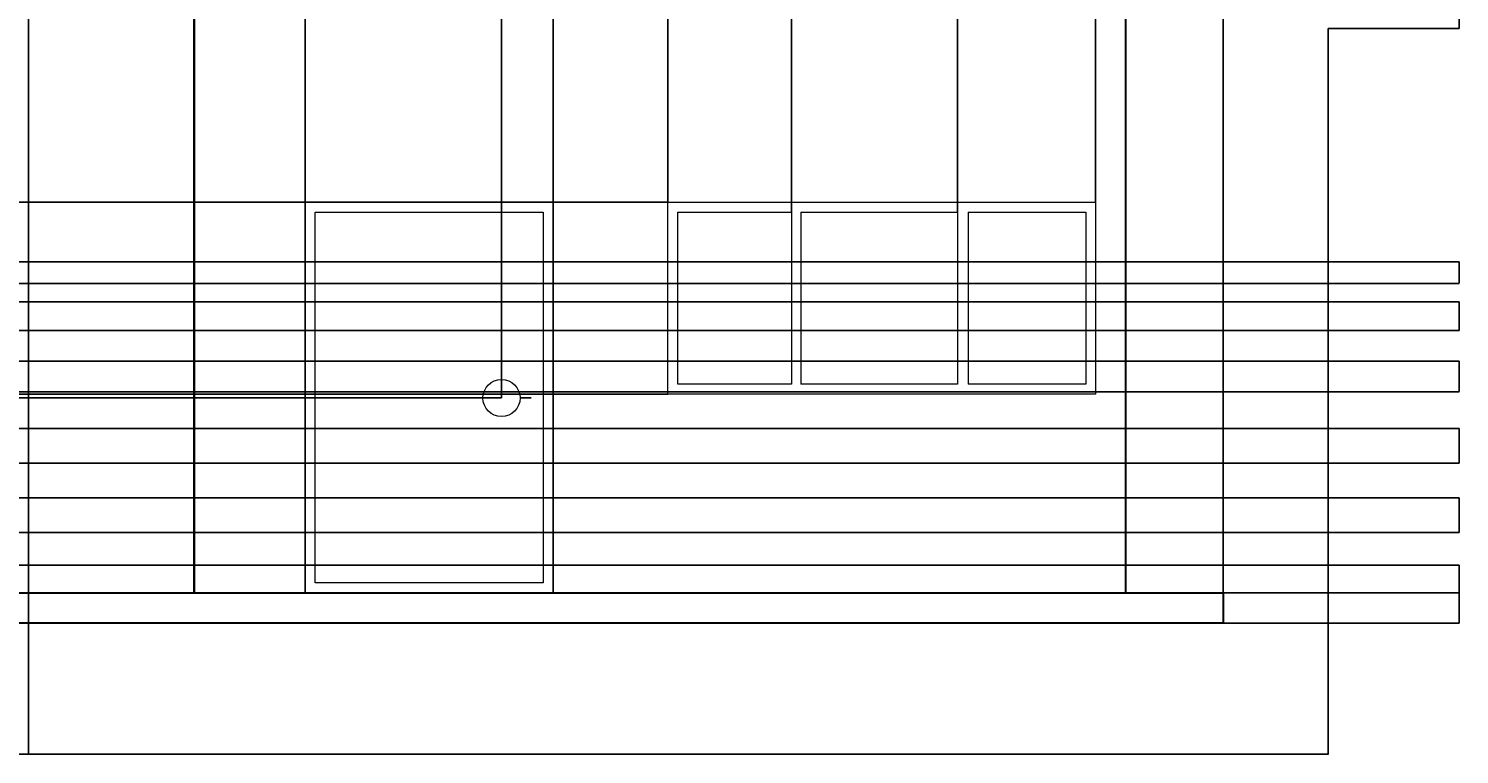
# Model space of a CAD drawing. Units: millimetres. Extents: x 1225 to 9865, y 11 to 4912.
# Tile 3 of 4: x 5562 to 9865, y 11 to 2192. Entities that reach past the tile are written whole.
import ezdxf

# ---------------------------------------------------------------- set-up
doc = ezdxf.new("R2010")
doc.units = ezdxf.units.MM
for name, color, linetype, lineweight in [('A-ANNO-DIMS', 2, 'Continuous', 18), ('A-COLS', 7, 'Continuous', 35), ('A-DOOR', 3, 'Continuous', 20), ('A-GLAZ', 4, 'Continuous', 18), ('A-WALL', 7, 'Continuous', 30), ('S-FNDN', 7, 'Continuous', 30)]:
    doc.layers.add(name, color=color, linetype=linetype, lineweight=lineweight)
doc.styles.get("Standard").update_dxf_attribs({"font": 'arial.ttf'})
doc.dimstyles.get("Standard").update_dxf_attribs({"dimtxt": 0.18, "dimasz": 0.18, "dimexe": 0.18, "dimexo": 0.0625, "dimgap": 0.09, "dimtad": 0, "dimtih": 1, "dimtoh": 1, "dimdec": 4, "dimzin": 0, "dimdsep": 46, "dimtxsty": 'Standard', "dimcen": 0.09, "dimadec": 0, "dimazin": 0, "dimtfac": 1, "dimtdec": 4, "dimtofl": 0, "dimtmove": 0, "dimatfit": 3, "dimfxl": 1, "dimtolj": 1, "dimtzin": 0, "dimarcsym": 0})

# ---------------------------------------------------------------- blocks, each defined once
blk = doc.blocks.new('*D1')
at = {"layer": 'A-ANNO-DIMS', "color": 0, "lineweight": -2, "transparency": 16777216}
for p, q in [((9470.3, 2192.1), (9470.3, 10.6)), ((1619.2, 404.7), (1619.2, 10.6)), ((1619.3, 10.8), (5544.4, 10.8)), ((9470.1, 10.8), (5545.1, 10.8))]:
    blk.add_line(p, q, dxfattribs=at)
at = {"layer": 'A-ANNO-DIMS', "color": 0, "transparency": 16777216}
for points in [[(1619.3, 10.8), (1619.3, 10.7), (1619.2, 10.8)], [(9470.1, 10.8), (9470.1, 10.7), (9470.3, 10.8)]]:
    blk.add_solid(points, dxfattribs=at)
at = {"layer": 'Defpoints', "color": 0, "transparency": 16777216}
for p in [(9470.3, 2192.2), (1619.2, 404.8), (9470.3, 10.8)]:
    blk.add_point(p, dxfattribs=at)
at = {"layer": 'A-ANNO-DIMS', "color": 0, "transparency": 16777216, "insert": (5544.7, 10.8), "char_height": 0.18, "attachment_point": 5}
blk.add_mtext('\\A1;7851', dxfattribs=at)
blk = doc.blocks.new('*D9')
at = {"layer": 'A-ANNO-DIMS', "color": 0, "lineweight": -2, "transparency": 16777216}
for p, q in [((5415.4, 4322.4), (5415.4, 10.6)), ((5561.8, 4322.4), (5561.8, 10.6)), ((5415.6, 10.8), (5488.1, 10.8)), ((5561.6, 10.8), (5489, 10.8))]:
    blk.add_line(p, q, dxfattribs=at)
at = {"layer": 'A-ANNO-DIMS', "color": 0, "transparency": 16777216}
for points in [[(5415.6, 10.8), (5415.6, 10.7), (5415.4, 10.8)], [(5561.6, 10.8), (5561.6, 10.7), (5561.8, 10.8)]]:
    blk.add_solid(points, dxfattribs=at)
at = {"layer": 'Defpoints', "color": 0, "transparency": 16777216}
for p in [(5415.4, 4322.4), (5561.8, 4322.4), (5561.8, 10.8)]:
    blk.add_point(p, dxfattribs=at)
at = {"layer": 'A-ANNO-DIMS', "color": 0, "transparency": 16777216, "insert": (5488.6, 10.8), "char_height": 0.18, "attachment_point": 5}
blk.add_mtext('\\A1;146.38', dxfattribs=at)
blk = doc.blocks.new('*D12')
at = {"layer": 'A-ANNO-DIMS', "color": 0, "lineweight": -2, "transparency": 16777216}
for p, q in [((6059.9, 496.3), (6059.9, 4911.8)), ((6060.1, 4911.6), (6226, 4911.6)), ((6392.9, 4911.6), (6226.9, 4911.6)), ((6393.1, 496.3), (6393.1, 4911.8))]:
    blk.add_line(p, q, dxfattribs=at)
at = {"layer": 'A-ANNO-DIMS', "color": 0, "transparency": 16777216}
for points in [[(6060.1, 4911.6), (6060.1, 4911.6), (6059.9, 4911.6)], [(6392.9, 4911.6), (6392.9, 4911.6), (6393.1, 4911.6)]]:
    blk.add_solid(points, dxfattribs=at)
at = {"layer": 'Defpoints', "color": 0, "transparency": 16777216}
for p in [(6393.1, 4911.6), (6059.9, 496.3), (6393.1, 496.3)]:
    blk.add_point(p, dxfattribs=at)
at = {"layer": 'A-ANNO-DIMS', "color": 0, "transparency": 16777216, "insert": (6226.5, 4911.6), "char_height": 0.18, "attachment_point": 5}
blk.add_mtext('\\A1;333.14', dxfattribs=at)
blk = doc.blocks.new('*D13')
at = {"layer": 'A-ANNO-DIMS', "color": 0, "lineweight": -2, "transparency": 16777216}
for p, q in [((6393.1, 1670.9), (6393.1, 4911.8)), ((6393.2, 4911.6), (6765.6, 4911.6)), ((7138.7, 4911.6), (6766.3, 4911.6)), ((7138.8, 1670.9), (7138.8, 4911.8))]:
    blk.add_line(p, q, dxfattribs=at)
at = {"layer": 'A-ANNO-DIMS', "color": 0, "transparency": 16777216}
for points in [[(6393.2, 4911.6), (6393.2, 4911.6), (6393.1, 4911.6)], [(7138.7, 4911.6), (7138.7, 4911.6), (7138.8, 4911.6)]]:
    blk.add_solid(points, dxfattribs=at)
at = {"layer": 'Defpoints', "color": 0, "transparency": 16777216}
for p in [(7138.8, 4911.6), (6393.1, 1670.8), (7138.8, 1670.8)]:
    blk.add_point(p, dxfattribs=at)
at = {"layer": 'A-ANNO-DIMS', "color": 0, "transparency": 16777216, "insert": (6765.9, 4911.6), "char_height": 0.18, "attachment_point": 5}
blk.add_mtext('\\A1;745.8', dxfattribs=at)
blk = doc.blocks.new('*D14')
at = {"layer": 'A-ANNO-DIMS', "color": 0, "lineweight": -2, "transparency": 16777216}
for p, q in [((6983.8, 1082), (6983.8, 4911.8)), ((6984, 4911.6), (7061.1, 4911.6)), ((7138.7, 4911.6), (7061.6, 4911.6)), ((7138.8, 496.3), (7138.8, 4911.8))]:
    blk.add_line(p, q, dxfattribs=at)
at = {"layer": 'A-ANNO-DIMS', "color": 0, "transparency": 16777216}
for points in [[(6984, 4911.6), (6984, 4911.6), (6983.8, 4911.6)], [(7138.7, 4911.6), (7138.7, 4911.6), (7138.8, 4911.6)]]:
    blk.add_solid(points, dxfattribs=at)
at = {"layer": 'Defpoints', "color": 0, "transparency": 16777216}
for p in [(7138.8, 4911.6), (6983.8, 1081.9), (7138.8, 496.3)]:
    blk.add_point(p, dxfattribs=at)
at = {"layer": 'A-ANNO-DIMS', "color": 0, "transparency": 16777216, "insert": (7061.3, 4911.6), "char_height": 0.18, "attachment_point": 5}
blk.add_mtext('\\A1;155', dxfattribs=at)
blk = doc.blocks.new('*D15')
at = {"layer": 'A-ANNO-DIMS', "color": 0, "lineweight": -2, "transparency": 16777216}
for p, q in [((7138.8, 1670.9), (7138.8, 4911.8)), ((7139, 4911.6), (7311.1, 4911.6)), ((7484.1, 4911.6), (7311.9, 4911.6)), ((7484.2, 1670.9), (7484.2, 4911.8))]:
    blk.add_line(p, q, dxfattribs=at)
at = {"layer": 'A-ANNO-DIMS', "color": 0, "transparency": 16777216}
for points in [[(7139, 4911.6), (7139, 4911.6), (7138.8, 4911.6)], [(7484.1, 4911.6), (7484.1, 4911.6), (7484.2, 4911.6)]]:
    blk.add_solid(points, dxfattribs=at)
at = {"layer": 'Defpoints', "color": 0, "transparency": 16777216}
for p in [(7484.2, 4911.6), (7138.8, 1670.8), (7484.2, 1670.8)]:
    blk.add_point(p, dxfattribs=at)
at = {"layer": 'A-ANNO-DIMS', "color": 0, "transparency": 16777216, "insert": (7311.5, 4911.6), "char_height": 0.18, "attachment_point": 5}
blk.add_mtext('\\A1;345.4', dxfattribs=at)
blk = doc.blocks.new('*D16')
at = {"layer": 'A-ANNO-DIMS', "color": 0, "lineweight": -2, "transparency": 16777216}
for p, q in [((8861.3, 496.3), (8861.3, 4911.8)), ((8861.4, 4911.6), (9007.3, 4911.6)), ((9153.9, 4911.6), (9008.1, 4911.6)), ((9154.1, 496.3), (9154.1, 4911.8))]:
    blk.add_line(p, q, dxfattribs=at)
at = {"layer": 'A-ANNO-DIMS', "color": 0, "transparency": 16777216}
for points in [[(8861.4, 4911.6), (8861.4, 4911.6), (8861.3, 4911.6)], [(9153.9, 4911.6), (9153.9, 4911.6), (9154.1, 4911.6)]]:
    blk.add_solid(points, dxfattribs=at)
at = {"layer": 'Defpoints', "color": 0, "transparency": 16777216}
for p in [(9154.1, 4911.6), (8861.3, 496.3), (9154.1, 496.3)]:
    blk.add_point(p, dxfattribs=at)
at = {"layer": 'A-ANNO-DIMS', "color": 0, "transparency": 16777216, "insert": (9007.7, 4911.6), "char_height": 0.18, "attachment_point": 5}
blk.add_mtext('\\A1;292.8', dxfattribs=at)
blk = doc.blocks.new('*D26')
at = {"layer": 'A-ANNO-DIMS', "color": 0, "lineweight": -2, "transparency": 16777216}
for p, q in [((9154.1, 496.3), (9864.4, 496.3)), ((9864.3, 496.1), (9864.3, 450.7)), ((9864.3, 404.9), (9864.3, 450.3)), ((9154.1, 404.8), (9864.4, 404.8))]:
    blk.add_line(p, q, dxfattribs=at)
at = {"layer": 'A-ANNO-DIMS', "color": 0, "transparency": 16777216}
for points in [[(9864.2, 496.1), (9864.3, 496.1), (9864.3, 496.3)], [(9864.2, 404.9), (9864.3, 404.9), (9864.3, 404.8)]]:
    blk.add_solid(points, dxfattribs=at)
at = {"layer": 'Defpoints', "color": 0, "transparency": 16777216}
for p in [(9154.1, 496.3), (9864.3, 496.3), (9154.1, 404.8)]:
    blk.add_point(p, dxfattribs=at)
at = {"layer": 'A-ANNO-DIMS', "color": 0, "transparency": 16777216, "insert": (9864.3, 450.5), "char_height": 0.18, "attachment_point": 5}
blk.add_mtext('\\A1;91.51', dxfattribs=at)
blk = doc.blocks.new('*D30')
at = {"layer": 'A-ANNO-DIMS', "color": 0, "lineweight": -2, "transparency": 16777216}
for p, q in [((9470.3, 2343), (9864.4, 2343)), ((9864.3, 2342.8), (9864.3, 2267.8)), ((9864.3, 2192.3), (9864.3, 2267.4)), ((9470.3, 2192.2), (9864.4, 2192.2))]:
    blk.add_line(p, q, dxfattribs=at)
at = {"layer": 'A-ANNO-DIMS', "color": 0, "transparency": 16777216}
for points in [[(9864.2, 2342.8), (9864.3, 2342.8), (9864.3, 2343)], [(9864.2, 2192.3), (9864.3, 2192.3), (9864.3, 2192.2)]]:
    blk.add_solid(points, dxfattribs=at)
at = {"layer": 'Defpoints', "color": 0, "transparency": 16777216}
for p in [(9470.3, 2343), (9864.3, 2343), (9470.3, 2192.2)]:
    blk.add_point(p, dxfattribs=at)
at = {"layer": 'A-ANNO-DIMS', "color": 0, "transparency": 16777216, "insert": (9864.3, 2267.6), "char_height": 0.18, "attachment_point": 5}
blk.add_mtext('\\A1;150.8', dxfattribs=at)
blk = doc.blocks.new('*D38')
at = {"layer": 'A-ANNO-DIMS', "color": 0, "lineweight": -2, "transparency": 16777216}
for p, q in [((6393, 1670.8), (1225, 1670.8)), ((1225.2, 1670.7), (1225.2, 1083.7)), ((1225.2, 496.4), (1225.2, 1083.4)), ((6393, 496.3), (1225, 496.3))]:
    blk.add_line(p, q, dxfattribs=at)
at = {"layer": 'A-ANNO-DIMS', "color": 0, "transparency": 16777216}
for points in [[(1225.1, 1670.7), (1225.2, 1670.7), (1225.2, 1670.8)], [(1225.1, 496.4), (1225.2, 496.4), (1225.2, 496.3)]]:
    blk.add_solid(points, dxfattribs=at)
at = {"layer": 'Defpoints', "color": 0, "transparency": 16777216}
for p in [(1225.2, 1670.8), (6393.1, 1670.8), (6393.1, 496.3)]:
    blk.add_point(p, dxfattribs=at)
at = {"layer": 'A-ANNO-DIMS', "color": 0, "transparency": 16777216, "insert": (1225.2, 1083.6), "char_height": 0.18, "attachment_point": 5}
blk.add_mtext('\\A1;1174.6', dxfattribs=at)
blk = doc.blocks.new('*D39')
at = {"layer": 'A-ANNO-DIMS', "color": 0, "lineweight": -2, "transparency": 16777216}
for p, q in [((7484.2, 1670.8), (1225, 1670.8)), ((1225.2, 1670.7), (1225.2, 1382.4)), ((1225.2, 1093.8), (1225.2, 1382.1)), ((7484.2, 1093.7), (1225, 1093.7))]:
    blk.add_line(p, q, dxfattribs=at)
at = {"layer": 'A-ANNO-DIMS', "color": 0, "transparency": 16777216}
for points in [[(1225.1, 1670.7), (1225.2, 1670.7), (1225.2, 1670.8)], [(1225.1, 1093.8), (1225.2, 1093.8), (1225.2, 1093.7)]]:
    blk.add_solid(points, dxfattribs=at)
at = {"layer": 'Defpoints', "color": 0, "transparency": 16777216}
for p in [(1225.2, 1670.8), (7484.2, 1670.8), (7484.2, 1093.7)]:
    blk.add_point(p, dxfattribs=at)
at = {"layer": 'A-ANNO-DIMS', "color": 0, "transparency": 16777216, "insert": (1225.2, 1382.3), "char_height": 0.18, "attachment_point": 5}
blk.add_mtext('\\A1;577.2', dxfattribs=at)
blk = doc.blocks.new('*D44')
at = {"layer": 'A-ANNO-DIMS', "color": 0, "lineweight": -2, "transparency": 16777216}
for p, q in [((6983.8, 1081.9), (1225, 1081.9)), ((1225.2, 1081.8), (1225.2, 789.3)), ((1225.2, 496.4), (1225.2, 788.9)), ((7138.8, 496.3), (1225, 496.3))]:
    blk.add_line(p, q, dxfattribs=at)
at = {"layer": 'A-ANNO-DIMS', "color": 0, "transparency": 16777216}
for points in [[(1225.1, 1081.8), (1225.2, 1081.8), (1225.2, 1081.9)], [(1225.1, 496.4), (1225.2, 496.4), (1225.2, 496.3)]]:
    blk.add_solid(points, dxfattribs=at)
at = {"layer": 'Defpoints', "color": 0, "transparency": 16777216}
for p in [(6983.8, 1081.9), (1225.2, 496.3), (7138.8, 496.3)]:
    blk.add_point(p, dxfattribs=at)
at = {"layer": 'A-ANNO-DIMS', "color": 0, "transparency": 16777216, "insert": (1225.2, 789.1), "char_height": 0.18, "attachment_point": 5}
blk.add_mtext('\\A1;585.7', dxfattribs=at)
blk = doc.blocks.new('*D52')
at = {"layer": 'A-ANNO-DIMS', "color": 0, "lineweight": -2, "transparency": 16777216}
for p, q in [((7484.2, 1670.9), (7484.2, 4911.8)), ((7484.4, 4911.6), (7670, 4911.6)), ((7856.1, 4911.6), (7670.5, 4911.6)), ((7856.2, 1640.9), (7856.2, 4911.8))]:
    blk.add_line(p, q, dxfattribs=at)
at = {"layer": 'A-ANNO-DIMS', "color": 0, "transparency": 16777216}
for points in [[(7484.4, 4911.6), (7484.4, 4911.6), (7484.2, 4911.6)], [(7856.1, 4911.6), (7856.1, 4911.6), (7856.2, 4911.6)]]:
    blk.add_solid(points, dxfattribs=at)
at = {"layer": 'Defpoints', "color": 0, "transparency": 16777216}
for p in [(7856.2, 4911.6), (7484.2, 1670.8), (7856.2, 1640.8)]:
    blk.add_point(p, dxfattribs=at)
at = {"layer": 'A-ANNO-DIMS', "color": 0, "transparency": 16777216, "insert": (7670.2, 4911.6), "char_height": 0.18, "attachment_point": 5}
blk.add_mtext('\\A1;372', dxfattribs=at)
blk = doc.blocks.new('*D53')
at = {"layer": 'A-ANNO-DIMS', "color": 0, "lineweight": -2, "transparency": 16777216}
for p, q in [((7856.2, 1640.9), (7856.2, 4911.8)), ((7856.4, 4911.6), (8105.4, 4911.6)), ((8355.2, 4911.6), (8106.2, 4911.6)), ((8355.4, 1640.9), (8355.4, 4911.8))]:
    blk.add_line(p, q, dxfattribs=at)
at = {"layer": 'A-ANNO-DIMS', "color": 0, "transparency": 16777216}
for points in [[(7856.4, 4911.6), (7856.4, 4911.6), (7856.2, 4911.6)], [(8355.2, 4911.6), (8355.2, 4911.6), (8355.4, 4911.6)]]:
    blk.add_solid(points, dxfattribs=at)
at = {"layer": 'Defpoints', "color": 0, "transparency": 16777216}
for p in [(8355.4, 4911.6), (7856.2, 1640.8), (8355.4, 1640.8)]:
    blk.add_point(p, dxfattribs=at)
at = {"layer": 'A-ANNO-DIMS', "color": 0, "transparency": 16777216, "insert": (8105.8, 4911.6), "char_height": 0.18, "attachment_point": 5}
blk.add_mtext('\\A1;499.1', dxfattribs=at)
blk = doc.blocks.new('*D54')
at = {"layer": 'A-ANNO-DIMS', "color": 0, "lineweight": -2, "transparency": 16777216}
for p, q in [((8355.4, 1640.9), (8355.4, 4911.8)), ((8355.5, 4911.6), (8562.6, 4911.6)), ((8770.5, 4911.6), (8563.5, 4911.6)), ((8770.7, 1670.9), (8770.7, 4911.8))]:
    blk.add_line(p, q, dxfattribs=at)
at = {"layer": 'A-ANNO-DIMS', "color": 0, "transparency": 16777216}
for points in [[(8355.5, 4911.6), (8355.5, 4911.6), (8355.4, 4911.6)], [(8770.5, 4911.6), (8770.5, 4911.6), (8770.7, 4911.6)]]:
    blk.add_solid(points, dxfattribs=at)
at = {"layer": 'Defpoints', "color": 0, "transparency": 16777216}
for p in [(8770.7, 4911.6), (8355.4, 1640.8), (8770.7, 1670.8)]:
    blk.add_point(p, dxfattribs=at)
at = {"layer": 'A-ANNO-DIMS', "color": 0, "transparency": 16777216, "insert": (8563, 4911.6), "char_height": 0.18, "attachment_point": 5}
blk.add_mtext('\\A1;415.36', dxfattribs=at)
blk = doc.blocks.new('*D67')
at = {"layer": 'A-ANNO-DIMS', "color": 0, "lineweight": -2, "transparency": 16777216}
for p, q in [((4013.7, 579.2), (9864.4, 579.2)), ((9864.3, 579), (9864.3, 537.9)), ((9864.3, 496.4), (9864.3, 537.6)), ((4013.7, 496.3), (9864.4, 496.3))]:
    blk.add_line(p, q, dxfattribs=at)
at = {"layer": 'A-ANNO-DIMS', "color": 0, "transparency": 16777216}
for points in [[(9864.2, 579), (9864.3, 579), (9864.3, 579.2)], [(9864.2, 496.4), (9864.3, 496.4), (9864.3, 496.3)]]:
    blk.add_solid(points, dxfattribs=at)
at = {"layer": 'Defpoints', "color": 0, "transparency": 16777216}
for p in [(4013.6, 579.2), (9864.3, 579.2), (4013.6, 496.3)]:
    blk.add_point(p, dxfattribs=at)
at = {"layer": 'A-ANNO-DIMS', "color": 0, "transparency": 16777216, "insert": (9864.3, 537.7), "char_height": 0.18, "attachment_point": 5}
blk.add_mtext('\\A1;82.96', dxfattribs=at)
blk = doc.blocks.new('*D68')
at = {"layer": 'A-ANNO-DIMS', "color": 0, "lineweight": -2, "transparency": 16777216}
for p, q in [((4013.7, 781.7), (9864.4, 781.7)), ((9864.3, 781.5), (9864.3, 729.7)), ((9864.3, 677.6), (9864.3, 729.4)), ((4013.7, 677.4), (9864.4, 677.4))]:
    blk.add_line(p, q, dxfattribs=at)
at = {"layer": 'A-ANNO-DIMS', "color": 0, "transparency": 16777216}
for points in [[(9864.2, 781.5), (9864.3, 781.5), (9864.3, 781.7)], [(9864.2, 677.6), (9864.3, 677.6), (9864.3, 677.4)]]:
    blk.add_solid(points, dxfattribs=at)
at = {"layer": 'Defpoints', "color": 0, "transparency": 16777216}
for p in [(4013.6, 781.7), (9864.3, 781.7), (4013.6, 677.4)]:
    blk.add_point(p, dxfattribs=at)
at = {"layer": 'A-ANNO-DIMS', "color": 0, "transparency": 16777216, "insert": (9864.3, 729.5), "char_height": 0.18, "attachment_point": 5}
blk.add_mtext('\\A1;104.3', dxfattribs=at)
blk = doc.blocks.new('*D69')
at = {"layer": 'A-ANNO-DIMS', "color": 0, "lineweight": -2, "transparency": 16777216}
for p, q in [((4013.7, 990.3), (9864.4, 990.3)), ((9864.3, 990.1), (9864.3, 938.3)), ((9864.3, 886.2), (9864.3, 938)), ((4013.7, 886), (9864.4, 886))]:
    blk.add_line(p, q, dxfattribs=at)
at = {"layer": 'A-ANNO-DIMS', "color": 0, "transparency": 16777216}
for points in [[(9864.2, 990.1), (9864.3, 990.1), (9864.3, 990.3)], [(9864.2, 886.2), (9864.3, 886.2), (9864.3, 886)]]:
    blk.add_solid(points, dxfattribs=at)
at = {"layer": 'Defpoints', "color": 0, "transparency": 16777216}
for p in [(4013.6, 990.3), (9864.3, 990.3), (4013.6, 886)]:
    blk.add_point(p, dxfattribs=at)
at = {"layer": 'A-ANNO-DIMS', "color": 0, "transparency": 16777216, "insert": (9864.3, 938.2), "char_height": 0.18, "attachment_point": 5}
blk.add_mtext('\\A1;104.3', dxfattribs=at)
blk = doc.blocks.new('*D70')
at = {"layer": 'A-ANNO-DIMS', "color": 0, "lineweight": -2, "transparency": 16777216}
for p, q in [((4013.7, 1192.8), (9864.4, 1192.8)), ((9864.3, 1192.6), (9864.3, 1147)), ((9864.3, 1100.9), (9864.3, 1146.6)), ((4013.7, 1100.8), (9864.4, 1100.8))]:
    blk.add_line(p, q, dxfattribs=at)
at = {"layer": 'A-ANNO-DIMS', "color": 0, "transparency": 16777216}
for points in [[(9864.2, 1192.6), (9864.3, 1192.6), (9864.3, 1192.8)], [(9864.2, 1100.9), (9864.3, 1100.9), (9864.3, 1100.8)]]:
    blk.add_solid(points, dxfattribs=at)
at = {"layer": 'Defpoints', "color": 0, "transparency": 16777216}
for p in [(4013.6, 1192.8), (9864.3, 1192.8), (4013.6, 1100.8)]:
    blk.add_point(p, dxfattribs=at)
at = {"layer": 'A-ANNO-DIMS', "color": 0, "transparency": 16777216, "insert": (9864.3, 1146.8), "char_height": 0.18, "attachment_point": 5}
blk.add_mtext('\\A1;92.04', dxfattribs=at)
blk = doc.blocks.new('*D71')
at = {"layer": 'A-ANNO-DIMS', "color": 0, "lineweight": -2, "transparency": 16777216}
for p, q in [((4013.7, 1370.7), (9864.4, 1370.7)), ((9864.3, 1370.6), (9864.3, 1328)), ((9864.3, 1285), (9864.3, 1327.6)), ((4013.7, 1284.8), (9864.4, 1284.8))]:
    blk.add_line(p, q, dxfattribs=at)
at = {"layer": 'A-ANNO-DIMS', "color": 0, "transparency": 16777216}
for points in [[(9864.2, 1370.6), (9864.3, 1370.6), (9864.3, 1370.7)], [(9864.2, 1285), (9864.3, 1285), (9864.3, 1284.8)]]:
    blk.add_solid(points, dxfattribs=at)
at = {"layer": 'Defpoints', "color": 0, "transparency": 16777216}
for p in [(4013.6, 1370.7), (9864.3, 1370.7), (4013.6, 1284.8)]:
    blk.add_point(p, dxfattribs=at)
at = {"layer": 'A-ANNO-DIMS', "color": 0, "transparency": 16777216, "insert": (9864.3, 1327.8), "char_height": 0.18, "attachment_point": 5}
blk.add_mtext('\\A1;85.9', dxfattribs=at)
blk = doc.blocks.new('*D72')
at = {"layer": 'A-ANNO-DIMS', "color": 0, "lineweight": -2, "transparency": 16777216}
for p, q in [((4013.7, 1491.5), (9864.4, 1491.5)), ((9864.3, 1491.4), (9864.3, 1459.1)), ((4013.7, 1426.4), (9864.4, 1426.4)), ((9864.3, 1426.6), (9864.3, 1458.8))]:
    blk.add_line(p, q, dxfattribs=at)
at = {"layer": 'A-ANNO-DIMS', "color": 0, "transparency": 16777216}
for points in [[(9864.2, 1491.4), (9864.3, 1491.4), (9864.3, 1491.5)], [(9864.2, 1426.6), (9864.3, 1426.6), (9864.3, 1426.4)]]:
    blk.add_solid(points, dxfattribs=at)
at = {"layer": 'Defpoints', "color": 0, "transparency": 16777216}
for p in [(4013.6, 1491.5), (9864.3, 1491.5), (4013.6, 1426.4)]:
    blk.add_point(p, dxfattribs=at)
at = {"layer": 'A-ANNO-DIMS', "color": 0, "transparency": 16777216, "insert": (9864.3, 1459), "char_height": 0.18, "attachment_point": 5}
blk.add_mtext('\\A1;65.16', dxfattribs=at)
blk = doc.blocks.new('*D73')
at = {"layer": 'A-ANNO-DIMS', "color": 0, "lineweight": -2, "transparency": 16777216}
for p, q in [((6983.8, 1081.9), (6983.8, 1082)), ((6983.8, 1081.9), (6983.9, 1081.9)), ((7073.2, 1081.9), (7039.9, 1081.9))]:
    blk.add_line(p, q, dxfattribs=at)
at = {"layer": 'A-ANNO-DIMS', "color": 0, "transparency": 16777216}
blk.add_solid([(7039.9, 1082), (7039.9, 1081.9), (7039.7, 1081.9)], dxfattribs=at)
at = {"layer": 'Defpoints', "color": 0, "transparency": 16777216}
for p in [(6928, 1081.9), (7039.7, 1081.9)]:
    blk.add_point(p, dxfattribs=at)
at = {"layer": 'A-ANNO-DIMS', "color": 0, "transparency": 16777216, "insert": (7073.8, 1081.9), "char_height": 0.18, "attachment_point": 5}
blk.add_mtext('\\A1;∅111.74', dxfattribs=at)

msp = doc.modelspace()

# ---------------------------------------------------------------- linework, layer by layer
at = {"layer": 'A-COLS'}
msp.add_line((6059.917, 4517.596), (6059.917, 496.264), dxfattribs=at)
at = {"layer": 'A-DOOR'}
for points in [[(6393.055, 1670.836), (7138.844, 1670.836), (7138.844, 496.264), (6393.055, 496.264)], [(6423.055, 1640.836), (7108.844, 1640.836), (7108.844, 526.264), (6423.055, 526.264)]]:
    msp.add_lwpolyline(points, close=True, dxfattribs=at)
msp.add_circle((6983.847, 1081.944), 55.87, dxfattribs=at)
at = {"layer": 'A-GLAZ'}
for p, q in [((7856.234, 1640.836), (7856.234, 1123.666)), ((7884.302, 1640.836), (7884.302, 1123.666)), ((8355.362, 1640.836), (8355.362, 1123.666)), ((8387.1, 1640.836), (8387.1, 1123.666))]:
    msp.add_line(p, q, dxfattribs=at)
msp.add_lwpolyline([(7484.241, 1670.836), (8770.718, 1670.836), (8770.718, 1093.666), (7484.241, 1093.666)], close=True, dxfattribs=at)
for points in [[(7856.234, 1123.666), (7514.241, 1123.666), (7514.241, 1640.836), (7856.234, 1640.836)], [(7884.302, 1640.836), (8355.362, 1640.836)], [(8387.1, 1640.836), (8740.718, 1640.836), (8740.718, 1123.666), (8387.1, 1123.666)], [(8355.362, 1123.666), (7884.302, 1123.666)]]:
    msp.add_lwpolyline(points, dxfattribs=at)
at = {"layer": 'A-WALL'}
for p, q in [((8861.261, 496.264), (8861.261, 3844.439)), ((6059.917, 496.264), (8861.261, 496.264))]:
    msp.add_line(p, q, dxfattribs=at)
at = {"layer": 'S-FNDN'}
for p, q in [((1619.167, 496.264), (6462.269, 496.264)), ((6462.269, 496.264), (9154.083, 496.264)), ((9154.083, 496.264), (9154.083, 404.75)), ((6462.269, 404.75), (1619.167, 404.75)), ((9154.083, 404.75), (6462.269, 404.75))]:
    msp.add_line(p, q, dxfattribs=at)

# ---------------------------------------------------------------- dimensions: what is measured, and where the dimension line sits
at = {"layer": 'A-ANNO-DIMS'}
for base, p1, p2, override, picture, middle in [((6393.055, 4911.596), (6059.917, 496.264), (6393.055, 496.264), {"dimdec": 2, "dimlfac": 1, "dimrnd": 0, "dimzin": 0, "dimdsep": 46, "dimlunit": 2}, '*D12', (6226.486, 4911.596)), ((7138.844, 4911.596), (6393.055, 1670.836), (7138.844, 1670.836), {"dimdec": 1, "dimlfac": 1, "dimrnd": 0, "dimzin": 0, "dimdsep": 46, "dimlunit": 2}, '*D13', (6765.95, 4911.596)), ((7138.844, 4911.596), (6983.847, 1081.944), (7138.844, 496.264), {"dimdec": 0, "dimlfac": 1, "dimrnd": 0, "dimzin": 0, "dimdsep": 46, "dimlunit": 2}, '*D14', (7061.346, 4911.596)), ((7484.241, 4911.596), (7138.844, 1670.836), (7484.241, 1670.836), {"dimdec": 1, "dimlfac": 1, "dimrnd": 0, "dimzin": 0, "dimdsep": 46, "dimlunit": 2}, '*D15', (7311.543, 4911.596)), ((7856.234, 4911.596), (7484.241, 1670.836), (7856.234, 1640.836), {"dimdec": 0, "dimlfac": 1, "dimrnd": 0, "dimzin": 0, "dimdsep": 46, "dimlunit": 2}, '*D52', (7670.238, 4911.596)), ((8355.362, 4911.596), (7856.234, 1640.836), (8355.362, 1640.836), {"dimdec": 1, "dimlfac": 1, "dimrnd": 0, "dimzin": 0, "dimdsep": 46, "dimlunit": 2}, '*D53', (8105.798, 4911.596)), ((8770.718, 4911.596), (8355.362, 1640.836), (8770.718, 1670.836), {"dimdec": 2, "dimlfac": 1, "dimrnd": 0, "dimzin": 0, "dimdsep": 46, "dimlunit": 2}, '*D54', (8563.04, 4911.596)), ((9154.083, 4911.596), (8861.261, 496.264), (9154.083, 496.264), {"dimdec": 1, "dimlfac": 1, "dimrnd": 0, "dimzin": 0, "dimdsep": 46, "dimlunit": 2}, '*D16', (9007.672, 4911.596)), ((5561.752, 10.75), (5415.376, 4322.413), (5561.752, 4322.413), {"dimdec": 2, "dimlfac": 1, "dimrnd": 0, "dimzin": 0, "dimdsep": 46, "dimlunit": 2}, '*D9', (5488.564, 10.75)), ((9470.268, 10.75), (1619.167, 404.75), (9470.268, 2192.169), {"dimdec": 0, "dimlfac": 1, "dimrnd": 0, "dimzin": 0, "dimdsep": 46, "dimlunit": 2}, '*D1', (5544.717, 10.75))]:
    dim = msp.add_linear_dim(base=base, p1=p1, p2=p2, dimstyle='Standard', override=override, dxfattribs=at)
    dim.commit()
    dim.dimension.update_dxf_attribs({"geometry": picture, "text_midpoint": middle})
for base, p1, p2, override, picture, middle in [((9864.268, 2342.982), (9470.268, 2192.169), (9470.268, 2342.982), {"dimdec": 1, "dimlfac": 1, "dimrnd": 0, "dimzin": 0, "dimdsep": 46, "dimlunit": 2}, '*D30', (9864.268, 2267.576)), ((1225.167, 1670.836), (6393.055, 496.264), (6393.055, 1670.836), {"dimdec": 1, "dimlfac": 1, "dimrnd": 0, "dimzin": 0, "dimdsep": 46, "dimlunit": 2}, '*D38', (1225.167, 1083.55)), ((1225.167, 1670.836), (7484.241, 1093.666), (7484.241, 1670.836), {"dimdec": 1, "dimlfac": 1, "dimrnd": 0, "dimzin": 0, "dimdsep": 46, "dimlunit": 2}, '*D39', (1225.167, 1382.251)), ((9864.268, 1491.543), (4013.642, 1426.384), (4013.642, 1491.543), {"dimdec": 2, "dimlfac": 1, "dimrnd": 0, "dimzin": 0, "dimdsep": 46, "dimlunit": 2}, '*D72', (9864.268, 1458.964)), ((9864.268, 1370.736), (4013.642, 1284.835), (4013.642, 1370.736), {"dimdec": 1, "dimlfac": 1, "dimrnd": 0, "dimzin": 0, "dimdsep": 46, "dimlunit": 2}, '*D71', (9864.268, 1327.786)), ((9864.268, 1192.799), (4013.642, 1100.763), (4013.642, 1192.799), {"dimdec": 2, "dimlfac": 1, "dimrnd": 0, "dimzin": 0, "dimdsep": 46, "dimlunit": 2}, '*D70', (9864.268, 1146.781)), ((1225.167, 496.264), (6983.847, 1081.944), (7138.844, 496.264), {"dimdec": 1, "dimlfac": 1, "dimrnd": 0, "dimzin": 0, "dimdsep": 46, "dimlunit": 2}, '*D44', (1225.167, 789.104)), ((9864.268, 990.319), (4013.642, 886.011), (4013.642, 990.319), {"dimdec": 1, "dimlfac": 1, "dimrnd": 0, "dimzin": 0, "dimdsep": 46, "dimlunit": 2}, '*D69', (9864.268, 938.165)), ((9864.268, 781.703), (4013.642, 677.396), (4013.642, 781.703), {"dimdec": 1, "dimlfac": 1, "dimrnd": 0, "dimzin": 0, "dimdsep": 46, "dimlunit": 2}, '*D68', (9864.268, 729.549)), ((9864.268, 579.223), (4013.642, 496.264), (4013.642, 579.223), {"dimdec": 2, "dimlfac": 1, "dimrnd": 0, "dimzin": 0, "dimdsep": 46, "dimlunit": 2}, '*D67', (9864.268, 537.744)), ((9864.268, 496.264), (9154.083, 404.75), (9154.083, 496.264), {"dimdec": 2, "dimlfac": 1, "dimrnd": 0, "dimzin": 0, "dimdsep": 46, "dimlunit": 2}, '*D26', (9864.268, 450.507))]:
    dim = msp.add_linear_dim(base=base, p1=p1, p2=p2, angle=90, dimstyle='Standard', override=override, dxfattribs=at)
    dim.commit()
    dim.dimension.update_dxf_attribs({"geometry": picture, "text_midpoint": middle})
dim = msp.add_diameter_dim_2p(p1=(6927.977, 1081.944), p2=(7039.717, 1081.944), dimstyle='Standard', override={"dimdec": 2, "dimlfac": 1, "dimrnd": 0, "dimzin": 0, "dimdsep": 46, "dimlunit": 2}, dxfattribs=at)
dim.commit()
dim.dimension.update_dxf_attribs({"geometry": '*D73', "text_midpoint": (7073.24, 1081.944), "dimtype": 163})

doc.saveas('drawing.dxf')
